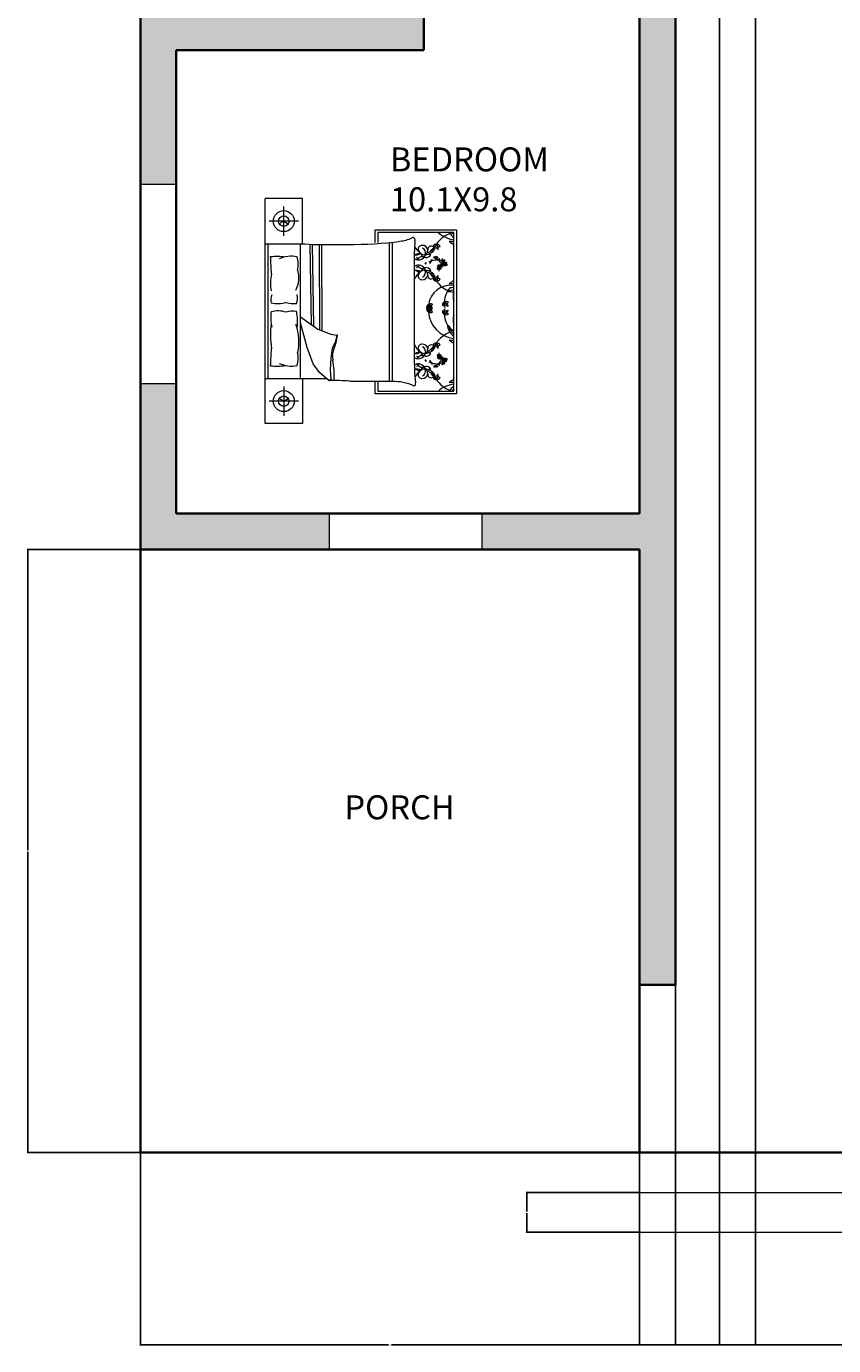
# Model space of a CAD drawing. Units: inches. Extents: x 8 to 486, y -516 to 97.
# Tile 1 of 5: x 9 to 211, y -516 to -185. Entities that reach past the tile are written whole.
import ezdxf

# ---------------------------------------------------------------- set-up
doc = ezdxf.new("R2010")
doc.units = ezdxf.units.IN
doc.header["$MEASUREMENT"] = 0
for name, color, linetype, lineweight in [('A-ANNO-DIMS', 2, 'Continuous', 18), ('A-AREA-IDEN', 7, 'Continuous', 18), ('A-FLOR-STRS', 7, 'Continuous', 18), ('A-FURN', 8, 'Continuous', 18), ('A-GLAZ', 4, 'Continuous', 18), ('A-WALL', 7, 'Continuous', 35), ('A-WALL-PATT', 150, 'Continuous', 13)]:
    doc.layers.add(name, color=color, linetype=linetype, lineweight=lineweight)
doc.styles.get("Standard").update_dxf_attribs({"font": 'arial.ttf'})
doc.dimstyles.get("Standard").update_dxf_attribs({"dimtxt": 0.18, "dimasz": 0.18, "dimexe": 0.18, "dimexo": 0.0625, "dimgap": 0.09, "dimtad": 0, "dimtih": 1, "dimtoh": 1, "dimdec": 0, "dimzin": 0, "dimdsep": 46, "dimlunit": 3, "dimtxsty": 'Standard', "dimcen": 0.09, "dimadec": 0, "dimazin": 0, "dimtfac": 1, "dimtdec": 0, "dimtofl": 0, "dimtmove": 0, "dimatfit": 3, "dimfxl": 1, "dimtolj": 1, "dimtzin": 0, "dimarcsym": 0})

# ---------------------------------------------------------------- blocks, each defined once
blk = doc.blocks.new('BED-DOUBLE')
for p, q in [((0, 0), (0, 56.34)), ((4.7, 47.03), (4.7, 54.39)), ((8.38, 50.71), (1.01, 50.71)), ((27.62, 45.39), (27.62, 48.51)), ((27.62, 48.51), (47.92, 48.51)), ((28.27, 47.86), (28.27, 45.37)), ((47.26, 47.86), (28.27, 47.86)), ((47.26, 8.09), (47.26, 47.86)), ((47.92, 48.51), (47.92, 7.44)), ((0.72, 45.07), (0.72, 11.27)), ((8.9, 11.27), (8.9, 45.07)), ((11.24, 44.92), (11.53, 24.86)), ((11.82, 44.9), (12.11, 24.44)), ((13.6, 44.87), (13.68, 23.48)), ((14.18, 44.87), (14.26, 23.26)), ((31.13, 45.33), (31.13, 10.62)), ((31.84, 45.38), (31.84, 10.62)), ((41.55, 42.31), (40.91, 42.43)), ((37.37, 39.61), (37.37, 16.73)), ((41.55, 38.37), (40.91, 38.24)), ((8.9, 26.75), (13.2, 23.66)), ((10.58, 19.09), (8.9, 25.24)), ((13.2, 23.66), (16.51, 22.4)), ((16.51, 22.4), (17.99, 22.17)), ((17.54, 20.35), (16.85, 18.87)), ((17.99, 22.17), (17.54, 20.35)), ((12.06, 14.99), (10.58, 19.09)), ((16.85, 18.87), (16.51, 16.36)), ((41.55, 17.58), (40.91, 17.7)), ((13.66, 12.82), (12.06, 14.99)), ((16.51, 16.36), (16.28, 13.5)), ((16.28, 13.5), (16.51, 11.22)), ((41.55, 13.64), (40.91, 13.52)), ((0, 11.27), (15.46, 11.27)), ((16.05, 10.76), (13.66, 12.82)), ((16.51, 11.22), (16.05, 10.76)), ((27.62, 7.44), (27.62, 10.62)), ((28.27, 10.62), (28.27, 8.09)), ((4.7, 9.31), (4.7, 1.95)), ((47.92, 7.44), (27.62, 7.44)), ((28.27, 8.09), (47.26, 8.09)), ((8.38, 5.63), (1.01, 5.63))]:
    blk.add_line(p, q)
for points in [[(0, 45.07), (9.39, 45.07), (9.39, 56.34), (0, 56.34)], [(4.7, 50.71), (3.56, 50.05)], [(4.7, 50.71), (5.83, 50.05)], [(9.39, 11.27), (9.39, 0), (0, 0)], [(4.7, 5.63), (3.56, 6.29)], [(4.7, 5.63), (5.83, 6.29)]]:
    blk.add_lwpolyline(points)
for points in [[(30.69, 45.31, 0.056112), (33.79, 45.72, 0.095341), (36.78, 46.51)], [(1.4, 41.84, -0.074897), (5.08, 41.77, 0.472817)], [(5.29, 30.31, -0.14099), (1.54, 30.2, -0.235245)], [(5.29, 27.91, 0.14099), (1.54, 28.02, 0.235245)], [(1.4, 14.5, 0.074897), (5.08, 14.57, -0.472817)], [(21.21, 10.65, 0.001242), (31.9, 10.62, -0.127202), (37.23, 9.49)]]:
    blk.add_lwpolyline(points, format="xyb")
for centre, radius in [((4.7, 50.71), 2.63), ((4.7, 50.71), 1.31), ((45.1, 39.99), 0.143), ((43.59, 39.05), 0.143), ((43.59, 16.9), 0.143), ((45.1, 15.96), 0.143), ((4.7, 5.63), 2.63), ((4.7, 5.63), 1.31)]:
    blk.add_circle(centre, radius)
for centre, radius, start, end in [((37.06, 46.09), 0.514, 336.5219, 123.8264), ((48.98, 40.75), 7.36, 111.4092, 145.6135), ((48.25, 53.34), 7.36, 228.1144, 262.255), ((49.24, 49.64), 3.59, 209.8884, 236.5383), ((49.91, 50.93), 4.47, 223.5186, 233.6964), ((15.79, 146.07), 101.24, 266.1, 270.9282), ((19.47, 176.89), 132.06, 269.1145, 274.8735), ((92.17, 41.33), 54.82, 175.2402, 181.8035), ((41.34, 46.16), 4.26, 203.6453, 236.3329), ((39.29, 43.68), 0.951, 88.9462, 185.5144), ((39.99, 43.97), 1.69, 193.079, 274.7067), ((39.43, 43.29), 1.35, 7.1143, 95.0551), ((38.92, 42.76), 1.31, 338.5779, 68.4181), ((39.13, 43.52), 1.64, 305.9599, 357.6409), ((39.73, 45.27), 2.66, 288.2955, 328.7386), ((41.6, 43.6), 0.846, 19.1312, 189.736), ((41.34, 43.8), 1.06, 285.6955, 4.031), ((42.75, 42.66), 1.12, 128.4175, 173.8338), ((42.51, 43.77), 0.518, 126.7319, 206.0245), ((42.76, 44.31), 0.61, 76.272, 177.0484), ((41.84, 45.56), 1.26, 284.7031, 328.6173), ((43.59, 43.96), 1.16, 125.7657, 194.5347), ((37.88, 46.02), 5.15, 332.8176, 347.4827), ((43.08, 44.11), 0.816, 20.9613, 102.2885), ((43.52, 44.92), 0.614, 181.7131, 301.5367), ((41.51, 43.68), 1.86, 2.0648, 41.1598), ((42.63, 44.37), 0.602, 316.2238, 62.3173), ((42.98, 44.02), 0.048, 20.2667, 316.2271), ((43.23, 43.75), 0.0444, 52.0591, 168.5166), ((43.28, 43.74), 0.0914, 168.5166, 2.0648), ((48.41, 47.64), 2.99, 221.0454, 247.4453), ((46.8, 55.83), 10.18, 266.3481, 272.5919), ((-534.78, 10.78), 537.08, 2.8502, 3.3148), ((6.56, 34.66), 7.26, 78.2417, 114.8684), ((0.75, 39.83), 7.55, 348.9631, 14.8961), ((37.99, 41.7), 0.679, 196.6343, 225.5483), ((37.79, 44.6), 2.33, 259.249, 301.1782), ((37.99, 41.7), 0.679, 127.675, 162.5814), ((38.39, 42.79), 1.8, 240.8249, 340.7178), ((37.86, 41.99), 0.843, 246.1646, 318.4347), ((38.39, 37.89), 1.8, 19.2822, 119.1751), ((38.8, 40.44), 2.17, 85.2696, 124.215), ((38.72, 43.06), 1.62, 240.0851, 262.564), ((39.35, 40.67), 1.16, 74.8529, 138.4347), ((40.34, 43), 1.4, 196.8663, 330.0915), ((39.75, 42.12), 0.35, 254.8529, 12.6959), ((38.8, 40.44), 2.17, 53.6555, 57.2989), ((40.21, 40.19), 0.177, 169.5864, 349.5616), ((39.95, 45.3), 3.02, 273.4924, 303.7117), ((40.28, 40.18), 0.109, 349.5616, 167.2949), ((43.11, 36.27), 4.67, 110.1059, 116.9968), ((41.55, 40.12), 0.296, 129.5056, 182.6421), ((40.7, 40.8), 0.89, 308.4388, 328.836), ((40.54, 41.53), 1.59, 296.5064, 305.3102), ((40.53, 40.71), 0.905, 336.3901, 344.4871), ((41.52, 40.48), 0.115, 83.9457, 185.6216), ((41.06, 40.58), 0.472, 328.836, 0.8141), ((41.3, 40.45), 0.27, 306.5232, 32.4668), ((41.62, 40.66), 0.115, 112.5583, 214.2343), ((41.55, 40.86), 0.27, 265.7131, 351.6568), ((41.31, 41.01), 0.472, 297.3659, 329.344), ((40.95, 41.42), 0.905, 313.6929, 321.7899), ((41.96, 40.8), 0.296, 115.5379, 168.6744), ((40.95, 41.22), 0.89, 329.344, 349.7412), ((43.11, 36.27), 4.67, 86.1723, 106.4158), ((40.24, 41.02), 1.59, 352.8698, 1.6736), ((42.35, 41.59), 0.111, 125.0752, 284.7644), ((42.52, 41.63), 0.239, 127.3642, 168.4363), ((42.33, 41.83), 0.345, 277.4968, 341.2737), ((42.6, 41.67), 0.137, 88.1325, 178.8919), ((42.88, 41.52), 0.297, 136.3462, 189.6513), ((42.71, 41.49), 0.124, 189.6513, 312.3208), ((42.74, 41.83), 0.143, 183.2768, 356.7232), ((43.19, 41.58), 0.47, 164.2829, 186.9148), ((42.63, 41.57), 0.235, 312.3208, 40.2111), ((43.13, 41.84), 0.333, 201.6382, 274.947), ((42.69, 41.38), 0.436, 42.3896, 66.5724), ((47.08, 44.83), 5.35, 217.9541, 226.8459), ((43, 41.64), 0.237, 10.9597, 52.2379), ((43.15, 41.62), 0.11, 274.947, 37.5263), ((43.38, 40.15), 0.654, 253.6301, 325.4631), ((43.56, 39.24), 0.463, 82.0748, 142.6895), ((43.52, 40.99), 0.115, 112.5583, 214.2343), ((43.45, 41.2), 0.27, 265.7131, 351.6568), ((43.21, 41.35), 0.472, 297.3659, 329.344), ((43.23, 38.6), 2.34, 60.7959, 85.244), ((38.25, 35.23), 7.7, 37.8256, 47.7588), ((42.85, 41.75), 0.905, 313.6929, 321.7899), ((43.52, 39.8), 0.398, 273.8774, 357.1501), ((43.85, 41.13), 0.296, 115.5379, 168.6744), ((42.85, 41.56), 0.89, 329.344, 349.7412), ((43.68, 40.08), 0.385, 262.0748, 308.2393), ((42.14, 41.35), 1.59, 352.8698, 1.6736), ((44.3, 39.69), 0.398, 181.4625, 249.4747), ((46.34, 38.35), 2.81, 130.182, 149.456), ((44.23, 40), 0.385, 215.1128, 261.2773), ((44.54, 39.98), 0.654, 197.889, 269.722), ((44.37, 41.03), 0.16, 33.0979, 123.1364), ((40.84, 38.77), 4.19, 31.1156, 34.8118), ((44.14, 40.76), 0.434, 2.3172, 70.5201), ((44.79, 39.95), 0.463, 139.3812, 199.9959), ((43.93, 40.29), 0.654, 310.9365, 22.7695), ((44.23, 40.25), 0.475, 285.6484, 332.2957), ((44.5, 40.65), 0.125, 135.7354, 318.1297), ((44.29, 40.86), 0.166, 315.7354, 31.1156), ((44.15, 40.5), 0.385, 319.3812, 5.5456), ((44.59, 40.65), 0.125, 68.2452, 250.6395), ((44.3, 40.81), 0.374, 352.6008, 57.1845), ((45.64, 38.3), 2.5, 111.7087, 116.2181), ((43.23, 38.6), 2.34, 47.5083, 55.9967), ((44.66, 40.89), 0.374, 252.8042, 349.6943), ((44.3, 40.22), 0.398, 331.1838, 51.6792), ((44.71, 39.75), 0.111, 125.0752, 284.7644), ((44.7, 40.92), 0.166, 248.2452, 323.6254), ((44.88, 39.79), 0.239, 93.635, 168.4363), ((44.55, 41.02), 0.434, 291.7087, 3.0299), ((44.85, 40.17), 0.141, 138.2946, 276.2474), ((44.69, 39.98), 0.345, 277.4968, 341.2737), ((44.9, 40.15), 0.196, 358.5719, 143.8954), ((41.46, 43.31), 4.19, 323.6254, 327.3216), ((44.97, 39.82), 0.137, 88.1325, 178.8919), ((45.02, 40.3), 0.197, 208.8493, 269.9355), ((44.85, 40.26), 0.226, 274.2123, 318.1587), ((45.24, 39.68), 0.297, 136.3462, 189.6513), ((44.89, 40.92), 0.16, 325.6077, 55.6462), ((45.55, 39.73), 0.47, 164.2829, 186.9148), ((45.54, 40.03), 0.452, 121.9501, 165.2442), ((45, 39.73), 0.235, 312.3208, 40.2111), ((45.5, 39.99), 0.333, 201.6382, 274.947), ((45.23, 40.2), 0.095, 262.868, 7.094), ((45.05, 39.54), 0.436, 42.3896, 66.5724), ((45.21, 40.28), 0.283, 278.5614, 22.5914), ((45.37, 39.79), 0.237, 10.9597, 118.7804), ((45.37, 40.29), 0.142, 44.3732, 121.9501), ((45.52, 39.77), 0.11, 274.947, 37.5263), ((11.26, 35.15), 9.9, 166.3427, 191.1841), ((1.3, 36.57), 7.17, 333.8761, 16.1746), ((37.99, 38.97), 0.679, 134.4517, 156.7144), ((37.99, 38.97), 0.679, 203.2856, 232.325), ((37.79, 36.08), 2.33, 58.8218, 100.2867), ((41.34, 34.52), 4.26, 123.6671, 158.5059), ((37.86, 38.68), 0.843, 41.5653, 113.8354), ((38.8, 40.23), 2.17, 235.785, 274.7304), ((38.72, 37.62), 1.62, 97.436, 119.9149), ((39.99, 36.71), 1.69, 85.2933, 166.921), ((39.29, 37), 0.951, 174.4856, 271.0538), ((39.35, 40.01), 1.16, 221.5653, 285.1471), ((40.34, 37.67), 1.4, 29.9085, 163.1337), ((39.43, 37.39), 1.35, 264.9449, 352.8857), ((38.92, 37.92), 1.31, 291.5819, 21.4221), ((39.75, 38.56), 0.35, 347.3041, 105.1471), ((38.8, 40.23), 2.17, 302.7011, 306.3445), ((39.13, 37.16), 1.64, 2.3591, 54.0401), ((39.95, 35.38), 3.02, 56.2883, 86.5076), ((39.73, 35.4), 2.66, 31.2614, 71.7045), ((41.6, 37.08), 0.846, 170.264, 340.8688), ((42.75, 38.01), 1.12, 186.1662, 231.5825), ((41.34, 36.88), 1.06, 355.969, 74.3045), ((42.51, 36.91), 0.518, 153.9755, 233.2681), ((43.59, 36.72), 1.16, 165.4653, 234.2343), ((37.88, 34.66), 5.15, 12.5173, 27.1824), ((41.51, 37), 1.86, 318.8402, 357.9352), ((42.63, 36.3), 0.602, 297.6827, 43.7762), ((43.52, 35.75), 0.614, 58.4633, 178.2869), ((43.01, 36.67), 0.0796, 43.7762, 339.7183), ((43.2, 38.81), 0.111, 125.0752, 284.7644), ((43.37, 38.85), 0.239, 93.635, 168.4363), ((43.51, 39.88), 0.475, 228.342, 274.9894), ((43.28, 36.93), 0.0914, 357.9352, 191.4834), ((43.23, 36.92), 0.0444, 191.4834, 307.9409), ((43.34, 39.23), 0.141, 138.2946, 276.2474), ((43.39, 39.21), 0.196, 358.5719, 143.8954), ((43.18, 39.05), 0.345, 277.4968, 341.2737), ((43.46, 38.88), 0.137, 88.1325, 178.8919), ((43.51, 39.36), 0.197, 208.8493, 269.9355), ((43.34, 39.32), 0.226, 274.2123, 318.1587), ((43.73, 38.74), 0.297, 136.3462, 189.6513), ((43.56, 38.71), 0.124, 189.6513, 312.3208), ((46.34, 38.35), 2.81, 175.2415, 182.8929), ((44.04, 38.79), 0.47, 164.2829, 186.9148), ((44.03, 39.09), 0.452, 121.9501, 165.2442), ((43.49, 38.79), 0.235, 312.3208, 40.2111), ((43.98, 39.06), 0.333, 201.6382, 274.947), ((43.71, 39.26), 0.095, 262.868, 7.094), ((43.54, 38.6), 0.436, 42.3896, 66.5724), ((43.7, 39.34), 0.283, 278.5614, 22.5914), ((43.86, 38.86), 0.237, 10.9597, 118.7804), ((46.34, 38.35), 2.81, 156.1523, 156.9499), ((43.86, 39.35), 0.142, 44.3732, 121.9501), ((44, 38.83), 0.11, 274.947, 37.5263), ((44.34, 39.76), 0.475, 248.3627, 295.0101), ((44.1, 39.16), 0.463, 20.6625, 81.2773), ((45.07, 39.65), 0.124, 189.6513, 312.3208), ((46.55, 28.98), 5.69, 82.8636, 171.8197), ((42.76, 36.36), 0.61, 182.9516, 283.728), ((41.84, 35.12), 1.26, 31.3827, 75.2969), ((43.08, 36.57), 0.816, 257.7115, 339.0387), ((48.98, 39.93), 7.36, 214.3865, 248.5908), ((52.19, 29.78), 7.36, 152.5854, 175.5377), ((46.95, 32.74), 1.32, 76.3898, 169.0739), ((46.77, 31.74), 1.67, 72.8609, 131.9049), ((48.41, 33.04), 2.99, 112.5547, 138.9546), ((46.8, 24.84), 10.18, 87.4081, 93.6519), ((4.21, 30.97), 2.79, 153.3437, 196.1026), ((7.17, 36.95), 6.9, 254.1707, 275.9871), ((5.19, 31.35), 2.99, 335.0183, 18.5407), ((41.09, 29.2), 0.61, 106.1963, 206.9726), ((39.66, 29.82), 1.26, 314.6273, 358.5415), ((41.98, 29.31), 1.16, 155.6899, 224.4589), ((41.47, 29.19), 0.816, 50.8855, 132.2127), ((41.44, 30.11), 0.614, 211.6373, 331.4609), ((40.94, 29.19), 0.602, 346.148, 92.2415), ((40.32, 28.03), 1.86, 31.989, 71.0841), ((36.01, 28.25), 5.15, 2.7418, 17.407), ((45.03, 29.77), 0.61, 106.1963, 206.9726), ((43.6, 30.38), 1.26, 314.6273, 358.5415), ((45.92, 29.87), 1.16, 155.6899, 224.4589), ((45.41, 29.75), 0.816, 50.8855, 132.2127), ((45.38, 30.68), 0.614, 211.6373, 331.4609), ((44.26, 28.59), 1.86, 31.989, 71.0841), ((39.95, 28.81), 5.15, 2.7418, 17.407), ((44.88, 29.75), 0.602, 346.148, 92.2415), ((46.03, 29.72), 3.29, 68.117, 96.6195), ((51.13, 31.84), 4.05, 162.9798, 196.4569), ((53.22, 30.24), 5.98, 174.3643, 175.6213), ((57.31, 27.08), 10.69, 160.0972, 160.2783), ((11.47, 26.54), 10.04, 171.5249, 193.96), ((7.17, 21.26), 6.9, 84.0129, 105.8293), ((-1.76, 25.79), 9.94, 349.8617, 13.6238), ((41.09, 28.62), 0.61, 153.0274, 253.8037), ((39.66, 28), 1.26, 1.4585, 45.3727), ((41.98, 28.51), 1.16, 135.5411, 204.3101), ((36.01, 29.58), 5.15, 342.593, 357.2582), ((40.32, 29.8), 1.86, 288.9159, 328.011), ((40.94, 28.64), 0.602, 267.7585, 13.852), ((41.44, 27.71), 0.614, 28.5391, 148.3627), ((41.47, 28.64), 0.816, 227.7873, 309.1145), ((48.25, 28.61), 7.36, 184.4623, 262.255), ((41.42, 29.06), 0.048, 50.1909, 346.0209), ((41.45, 28.76), 0.0796, 13.852, 309.9245), ((41.82, 28.97), 0.0914, 198.4408, 31.989), ((41.77, 28.95), 0.0444, 81.9833, 198.4408), ((41.82, 28.86), 0.0914, 328.011, 161.5592), ((41.77, 28.87), 0.0444, 161.5592, 278.0167), ((45.03, 28.06), 0.61, 153.0274, 253.8037), ((43.6, 27.44), 1.26, 1.4585, 45.3727), ((45.92, 27.95), 1.16, 135.5411, 204.3101), ((39.95, 29.01), 5.15, 342.593, 357.2582), ((44.26, 29.23), 1.86, 288.9159, 328.011), ((44.88, 28.07), 0.602, 267.7585, 13.852), ((45.38, 27.15), 0.614, 28.5391, 148.3627), ((45.41, 28.08), 0.816, 227.7873, 309.1145), ((52.19, 28.04), 7.36, 184.4623, 207.4146), ((45.36, 29.62), 0.048, 50.1909, 346.0209), ((45.39, 28.2), 0.0796, 13.852, 309.9245), ((45.76, 29.53), 0.0914, 198.4408, 31.989), ((45.71, 29.52), 0.0444, 81.9833, 198.4408), ((45.76, 28.3), 0.0914, 328.011, 161.5592), ((45.71, 28.31), 0.0444, 161.5592, 278.0167), ((51.13, 25.99), 4.05, 163.5431, 197.0202), ((53.22, 27.59), 5.98, 184.3787, 185.6357), ((57.31, 30.74), 10.69, 199.7217, 199.9028), ((21.79, 22.22), 20.43, 172.2196, 189.497), ((-4.62, 20.49), 13.1, 348.0397, 19.2615), ((49.24, 24.92), 3.59, 181.272, 236.5383), ((51.16, 28.56), 6.65, 214.0123, 234.053), ((49.91, 26.21), 4.47, 197.8504, 233.6964), ((-3.3, 26.09), 21.85, 340.1194, 349.3383), ((18.04, 22.05), 0.136, 358.8623, 109.7536), ((41.34, 21.43), 4.26, 201.4941, 236.3329), ((39.29, 18.95), 0.951, 88.9462, 185.5144), ((39.43, 18.56), 1.35, 7.1143, 95.0551), ((42.76, 19.58), 0.61, 76.272, 177.0484), ((41.84, 20.83), 1.26, 284.7031, 328.6173), ((43.59, 19.23), 1.16, 125.7657, 194.5347), ((37.88, 21.29), 5.15, 332.8176, 347.4827), ((48.98, 16.02), 7.36, 111.4092, 145.6135), ((43.08, 19.38), 0.816, 20.9613, 102.2885), ((42.63, 19.64), 0.602, 316.2238, 62.3173), ((41.51, 18.95), 1.86, 2.0648, 41.1598), ((43.52, 20.19), 0.614, 181.7131, 301.5367), ((46.8, 31.1), 10.18, 266.3481, 272.5919), ((48.41, 22.91), 2.99, 221.0454, 247.4453), ((-534.78, 45.56), 537.08, 356.6852, 357.1498), ((0.75, 16.51), 7.55, 345.1039, 11.0369), ((21.45, 16.81), 4.59, 156.2616, 191.3392), ((37.79, 19.87), 2.33, 259.7133, 301.1782), ((37.99, 16.98), 0.679, 127.675, 156.7144), ((96.02, 16.06), 58.65, 179.3433, 185.6887), ((37.99, 16.98), 0.679, 203.229, 225.5483), ((38.39, 18.06), 1.8, 240.8249, 340.7178), ((37.86, 17.26), 0.843, 246.1646, 318.4347), ((38.8, 15.72), 2.17, 85.2696, 124.215), ((38.72, 18.33), 1.62, 240.0851, 262.564), ((39.99, 19.24), 1.69, 193.079, 274.7067), ((39.35, 15.94), 1.16, 74.8529, 138.4347), ((40.34, 18.28), 1.4, 196.8663, 330.0915), ((38.92, 18.03), 1.31, 338.5779, 68.4181), ((39.75, 17.39), 0.35, 254.8529, 12.6959), ((38.8, 15.72), 2.17, 53.6555, 57.2989), ((39.13, 18.79), 1.64, 305.9599, 357.6409), ((39.95, 20.57), 3.02, 273.4924, 303.7117), ((39.73, 20.54), 2.66, 288.2955, 328.7386), ((41.6, 18.87), 0.846, 19.1312, 189.736), ((41.34, 19.07), 1.06, 285.6955, 4.031), ((42.75, 17.93), 1.12, 128.4175, 173.8338), ((42.51, 19.04), 0.518, 126.7319, 206.0245), ((42.98, 19.29), 0.048, 20.2667, 316.2271), ((43.2, 17.14), 0.111, 75.2356, 234.9248), ((43.37, 17.09), 0.239, 191.5637, 266.365), ((43.23, 19.02), 0.0444, 52.0591, 168.5166), ((43.28, 19.02), 0.0914, 168.5166, 2.0648), ((43.51, 16.07), 0.475, 85.0106, 131.658), ((43.34, 16.72), 0.141, 83.7526, 221.7054), ((43.18, 16.9), 0.345, 18.7263, 82.5032), ((43.39, 16.74), 0.196, 216.1046, 1.4281), ((43.46, 17.06), 0.137, 181.1081, 271.8675), ((43.51, 16.58), 0.197, 90.0645, 151.1507), ((43.34, 16.63), 0.226, 41.8413, 85.7877), ((43.73, 17.21), 0.297, 170.3487, 223.6538), ((43.56, 17.24), 0.124, 47.6792, 170.3487), ((46.34, 17.59), 2.81, 177.1071, 184.7585), ((43.52, 16.15), 0.398, 2.8499, 86.1226), ((44.04, 17.15), 0.47, 173.0852, 195.7171), ((44.03, 16.86), 0.452, 194.7558, 238.0499), ((43.49, 17.16), 0.235, 319.7889, 47.6792), ((43.98, 16.89), 0.333, 85.053, 158.3618), ((43.71, 16.68), 0.095, 352.906, 97.132), ((43.54, 17.35), 0.436, 293.4276, 317.6104), ((43.86, 17.09), 0.237, 241.2196, 349.0403), ((43.7, 16.6), 0.283, 337.4086, 81.4386), ((44.3, 16.26), 0.398, 110.5253, 178.5375), ((44.54, 15.97), 0.654, 90.278, 162.111), ((44, 17.11), 0.11, 322.4737, 85.053), ((44.34, 16.19), 0.475, 64.9899, 111.6373), ((44.1, 16.78), 0.463, 278.7227, 339.3375), ((6.56, 21.68), 7.26, 245.1316, 281.7583), ((-3.9, 11.73), 21.26, 357.4519, 11.3392), ((37.99, 14.24), 0.679, 134.4517, 153.558), ((37.99, 14.24), 0.679, 210.0293, 232.325), ((37.79, 11.35), 2.33, 58.8218, 99.1554), ((38.39, 13.16), 1.8, 19.2822, 119.1751), ((37.86, 13.96), 0.843, 41.5653, 113.8354), ((41.34, 9.79), 4.26, 123.6671, 153.2997), ((38.8, 15.5), 2.17, 235.785, 274.7304), ((38.72, 12.89), 1.62, 97.436, 119.9149), ((39.99, 11.98), 1.69, 85.2933, 166.921), ((39.35, 15.28), 1.16, 221.5653, 285.1471), ((40.34, 12.94), 1.4, 29.9085, 163.1337), ((38.92, 13.19), 1.31, 291.5819, 21.4221), ((39.75, 13.83), 0.35, 347.3041, 105.1471), ((38.8, 15.5), 2.17, 302.7011, 306.3445), ((40.21, 15.76), 0.177, 10.4384, 190.4136), ((39.13, 12.43), 1.64, 2.3591, 54.0401), ((39.95, 10.65), 3.02, 56.2883, 86.5076), ((40.28, 15.77), 0.109, 192.7051, 10.4384), ((43.11, 19.68), 4.67, 243.0032, 249.8941), ((40.7, 15.15), 0.89, 31.164, 51.5612), ((41.55, 15.83), 0.296, 177.3579, 230.4944), ((40.54, 14.42), 1.59, 54.6898, 63.4936), ((40.53, 15.24), 0.905, 15.5129, 23.6099), ((41.52, 15.47), 0.115, 174.3784, 276.0543), ((41.3, 15.5), 0.27, 327.5332, 53.4768), ((41.06, 15.36), 0.472, 359.1859, 31.164), ((41.62, 15.29), 0.115, 145.7657, 247.4417), ((41.55, 15.09), 0.27, 8.3432, 94.2869), ((41.31, 14.94), 0.472, 30.656, 62.6341), ((40.95, 14.53), 0.905, 38.2101, 46.3071), ((41.96, 15.15), 0.296, 191.3256, 244.4621), ((40.95, 14.72), 0.89, 10.2588, 30.656), ((43.11, 19.68), 4.67, 253.5842, 273.8277), ((40.24, 14.93), 1.59, 358.3264, 7.1302), ((42.35, 14.36), 0.111, 75.2356, 234.9248), ((42.52, 14.31), 0.239, 191.5637, 232.6358), ((42.33, 14.12), 0.345, 18.7263, 82.5032), ((42.6, 14.28), 0.137, 181.1081, 271.8675), ((42.88, 14.43), 0.297, 170.3487, 223.6538), ((42.71, 14.46), 0.124, 47.6792, 170.3487), ((42.74, 14.11), 0.143, 3.2768, 176.7232), ((43.19, 14.37), 0.47, 173.0852, 195.7171), ((42.63, 14.37), 0.235, 319.7889, 47.6792), ((43.13, 14.11), 0.333, 85.053, 158.3618), ((42.69, 14.57), 0.436, 293.4276, 317.6104), ((47.08, 11.12), 5.35, 133.1541, 142.0459), ((43, 14.31), 0.237, 307.7621, 349.0403), ((43.15, 14.33), 0.11, 322.4737, 85.053), ((43.38, 15.8), 0.654, 34.5369, 106.3699), ((43.56, 16.71), 0.463, 217.3105, 277.9252), ((43.52, 14.96), 0.115, 145.7657, 247.4417), ((38.25, 20.72), 7.7, 312.2412, 322.1744), ((43.23, 17.35), 2.34, 274.756, 299.2041), ((43.45, 14.75), 0.27, 8.3432, 94.2869), ((43.21, 14.6), 0.472, 30.656, 62.6341), ((42.85, 14.2), 0.905, 38.2101, 46.3071), ((43.85, 14.81), 0.296, 191.3256, 244.4621), ((42.85, 14.39), 0.89, 10.2588, 30.656), ((43.68, 15.87), 0.385, 51.7607, 97.9252), ((42.14, 14.59), 1.59, 358.3264, 7.1302), ((46.34, 17.59), 2.81, 203.0501, 203.8477), ((43.86, 16.59), 0.142, 238.0499, 315.6268), ((44.23, 15.95), 0.385, 98.7227, 144.8872), ((46.34, 17.59), 2.81, 210.544, 229.818), ((44.14, 15.19), 0.434, 289.4799, 357.6828), ((40.84, 17.17), 4.19, 325.1882, 328.8844), ((44.37, 14.91), 0.16, 236.8636, 326.9021), ((44.79, 15.99), 0.463, 160.0041, 220.6188), ((43.93, 15.66), 0.654, 337.2305, 49.0635), ((44.23, 15.7), 0.475, 27.7043, 74.3516), ((44.5, 15.3), 0.125, 41.8703, 224.2646), ((44.29, 15.09), 0.166, 328.8844, 44.2646), ((44.15, 15.44), 0.385, 354.4544, 40.6188), ((44.59, 15.29), 0.125, 109.3605, 291.7548), ((44.3, 15.14), 0.374, 302.8155, 7.3992), ((45.64, 17.65), 2.5, 243.7819, 248.2913), ((43.23, 17.35), 2.34, 304.0033, 312.4917), ((44.3, 15.72), 0.398, 308.3208, 28.8162), ((44.66, 15.06), 0.374, 10.3057, 107.1958), ((44.71, 16.2), 0.111, 75.2356, 234.9248), ((44.7, 15.02), 0.166, 36.3746, 111.7548), ((44.88, 16.16), 0.239, 191.5637, 266.365), ((44.85, 15.78), 0.141, 83.7526, 221.7054), ((44.55, 14.92), 0.434, 356.9701, 68.2913), ((44.69, 15.96), 0.345, 18.7263, 82.5032), ((44.9, 15.8), 0.196, 216.1046, 1.4281), ((44.97, 16.12), 0.137, 181.1081, 271.8675), ((41.46, 12.64), 4.19, 32.6784, 36.3746), ((45.02, 15.65), 0.197, 90.0645, 151.1507), ((44.85, 15.69), 0.226, 41.8413, 85.7877), ((45.07, 16.3), 0.124, 47.6792, 170.3487), ((45.24, 16.27), 0.297, 170.3487, 223.6538), ((44.89, 15.03), 0.16, 304.3538, 34.3923), ((45.55, 16.21), 0.47, 173.0852, 195.7171), ((45.54, 15.92), 0.452, 194.7558, 238.0499), ((45, 16.22), 0.235, 319.7889, 47.6792), ((45.5, 15.95), 0.333, 85.053, 158.3618), ((45.23, 15.75), 0.095, 352.906, 97.132), ((45.05, 16.41), 0.436, 293.4276, 317.6104), ((45.37, 16.15), 0.237, 241.2196, 349.0403), ((45.21, 15.67), 0.283, 337.4086, 81.4386), ((45.37, 15.66), 0.142, 238.0499, 315.6268), ((45.52, 16.18), 0.11, 322.4737, 85.053), ((17.45, -40.9), 51.68, 85.8294, 91.553), ((37.19, 10.01), 0.52, 273.98, 27.3412), ((39.29, 12.27), 0.951, 174.4856, 271.0538), ((39.43, 12.66), 1.35, 264.9449, 352.8857), ((39.73, 10.68), 2.66, 31.2614, 71.7045), ((41.6, 12.35), 0.846, 170.264, 340.8688), ((41.34, 12.15), 1.06, 355.969, 74.3045), ((42.75, 13.29), 1.12, 186.1662, 231.5825), ((42.51, 12.18), 0.518, 153.9755, 233.2681), ((41.84, 10.39), 1.26, 31.3827, 75.2969), ((42.76, 11.64), 0.61, 182.9516, 283.728), ((43.59, 11.99), 1.16, 165.4653, 234.2343), ((37.88, 9.93), 5.15, 12.5173, 27.1824), ((41.51, 12.27), 1.86, 318.8402, 357.9352), ((42.63, 11.58), 0.602, 297.6827, 43.7762), ((43.52, 11.03), 0.614, 58.4633, 178.2869), ((43.08, 11.84), 0.816, 257.7115, 339.0387), ((48.98, 15.2), 7.36, 214.3865, 248.5908), ((43.01, 11.94), 0.0796, 43.7762, 339.7183), ((43.28, 12.2), 0.0914, 357.9352, 191.4834), ((43.23, 12.2), 0.0444, 191.4834, 307.9409), ((48.41, 8.31), 2.99, 112.5547, 138.9546), ((46.8, 0.12), 10.18, 87.4081, 93.6519), ((48.25, 2.61), 7.36, 97.745, 131.8856), ((49.24, 6.3), 3.59, 123.4617, 150.1116), ((49.91, 5.01), 4.47, 126.3036, 136.4814)]:
    blk.add_arc(centre, radius, start, end)
blk = doc.blocks.new('*D21')
at = {"layer": 'A-ANNO-DIMS', "color": 0, "lineweight": -2, "transparency": 16777216}
for p, q in [((37.13, -467.33), (37.13, -515.64)), ((162.13, -467.33), (162.13, -515.64)), ((37.31, -515.46), (99.24, -515.46)), ((161.95, -515.46), (100.02, -515.46))]:
    blk.add_line(p, q, dxfattribs=at)
at = {"layer": 'A-ANNO-DIMS', "color": 0, "transparency": 16777216}
for points in [[(37.31, -515.43), (37.31, -515.49), (37.13, -515.46)], [(161.95, -515.43), (161.95, -515.49), (162.13, -515.46)]]:
    blk.add_solid(points, dxfattribs=at)
at = {"layer": 'Defpoints', "color": 0, "transparency": 16777216}
for p in [(37.13, -467.26), (162.13, -467.26), (162.13, -515.46)]:
    blk.add_point(p, dxfattribs=at)
at = {"layer": 'A-ANNO-DIMS', "color": 0, "transparency": 16777216, "insert": (99.63, -515.46), "char_height": 0.18, "attachment_point": 5}
blk.add_mtext('\\A1;10\'-5"', dxfattribs=at)
blk = doc.blocks.new('*D22')
at = {"layer": 'A-ANNO-DIMS', "color": 0, "lineweight": -2, "transparency": 16777216}
for p, q in [((162.13, -487.33), (162.13, -515.64)), ((294.01, -487.33), (294.01, -515.64)), ((162.31, -515.46), (227.68, -515.46)), ((293.83, -515.46), (228.46, -515.46))]:
    blk.add_line(p, q, dxfattribs=at)
at = {"layer": 'A-ANNO-DIMS', "color": 0, "transparency": 16777216}
for points in [[(162.31, -515.43), (162.31, -515.49), (162.13, -515.46)], [(293.83, -515.43), (293.83, -515.49), (294.01, -515.46)]]:
    blk.add_solid(points, dxfattribs=at)
at = {"layer": 'Defpoints', "color": 0, "transparency": 16777216}
for p in [(162.13, -487.26), (294.01, -487.26), (294.01, -515.46)]:
    blk.add_point(p, dxfattribs=at)
at = {"layer": 'A-ANNO-DIMS', "color": 0, "transparency": 16777216, "insert": (228.07, -515.46), "char_height": 0.18, "attachment_point": 5}
blk.add_mtext('\\A1;11\'-0"', dxfattribs=at)
blk = doc.blocks.new('*D24')
at = {"layer": 'A-ANNO-DIMS', "color": 0, "lineweight": -2, "transparency": 16777216}
for p, q in [((37.06, -316.26), (8.75, -316.26)), ((8.93, -316.44), (8.93, -391.58)), ((8.93, -467.08), (8.93, -391.95)), ((37.06, -467.26), (8.75, -467.26))]:
    blk.add_line(p, q, dxfattribs=at)
at = {"layer": 'A-ANNO-DIMS', "color": 0, "transparency": 16777216}
for points in [[(8.9, -316.44), (8.96, -316.44), (8.93, -316.26)], [(8.9, -467.08), (8.96, -467.08), (8.93, -467.26)]]:
    blk.add_solid(points, dxfattribs=at)
at = {"layer": 'Defpoints', "color": 0, "transparency": 16777216}
for p in [(37.13, -316.26), (8.93, -467.26), (37.13, -467.26)]:
    blk.add_point(p, dxfattribs=at)
at = {"layer": 'A-ANNO-DIMS', "color": 0, "transparency": 16777216, "insert": (8.93, -391.76), "char_height": 0.18, "attachment_point": 5}
blk.add_mtext('\\A1;12\'-7"', dxfattribs=at)
blk = doc.blocks.new('*D26')
at = {"layer": 'A-ANNO-DIMS', "color": 0, "lineweight": -2, "transparency": 16777216}
for p, q in [((162.06, -477.26), (133.75, -477.26)), ((133.93, -477.44), (133.93, -482.08)), ((133.93, -487.08), (133.93, -482.45)), ((162.06, -487.26), (133.75, -487.26))]:
    blk.add_line(p, q, dxfattribs=at)
at = {"layer": 'A-ANNO-DIMS', "color": 0, "transparency": 16777216}
for points in [[(133.9, -477.44), (133.96, -477.44), (133.93, -477.26)], [(133.9, -487.08), (133.96, -487.08), (133.93, -487.26)]]:
    blk.add_solid(points, dxfattribs=at)
at = {"layer": 'Defpoints', "color": 0, "transparency": 16777216}
for p in [(133.93, -477.26), (162.13, -477.26), (162.13, -487.26)]:
    blk.add_point(p, dxfattribs=at)
at = {"layer": 'A-ANNO-DIMS', "color": 0, "transparency": 16777216, "insert": (133.93, -482.26), "char_height": 0.18, "attachment_point": 5}
blk.add_mtext('\\A1;0\'-10"', dxfattribs=at)
blk = doc.blocks.new('*D34')
at = {"layer": 'A-ANNO-DIMS', "color": 0, "lineweight": -2, "transparency": 16777216}
for p, q in [((171.13, -425.33), (171.13, -515.64)), ((233.38, -425.33), (233.38, -515.64)), ((171.31, -515.46), (201.92, -515.46)), ((233.2, -515.46), (202.58, -515.46))]:
    blk.add_line(p, q, dxfattribs=at)
at = {"layer": 'A-ANNO-DIMS', "color": 0, "transparency": 16777216}
for points in [[(171.31, -515.43), (171.31, -515.49), (171.13, -515.46)], [(233.2, -515.43), (233.2, -515.49), (233.38, -515.46)]]:
    blk.add_solid(points, dxfattribs=at)
at = {"layer": 'Defpoints', "color": 0, "transparency": 16777216}
for p in [(171.13, -425.26), (233.38, -425.26), (233.38, -515.46)]:
    blk.add_point(p, dxfattribs=at)
at = {"layer": 'A-ANNO-DIMS', "color": 0, "transparency": 16777216, "insert": (202.25, -515.46), "char_height": 0.18, "attachment_point": 5}
blk.add_mtext('\\A1;5\'-2"', dxfattribs=at)
blk = doc.blocks.new('*D35')
at = {"layer": 'A-ANNO-DIMS', "color": 0, "lineweight": -2, "transparency": 16777216}
for p, q in [((182.13, -73.93), (182.13, -515.64)), ((191.13, -73.93), (191.13, -515.64)), ((182.31, -515.46), (186.3, -515.46)), ((190.95, -515.46), (186.96, -515.46))]:
    blk.add_line(p, q, dxfattribs=at)
at = {"layer": 'A-ANNO-DIMS', "color": 0, "transparency": 16777216}
for points in [[(182.31, -515.43), (182.31, -515.49), (182.13, -515.46)], [(190.95, -515.43), (190.95, -515.49), (191.13, -515.46)]]:
    blk.add_solid(points, dxfattribs=at)
at = {"layer": 'Defpoints', "color": 0, "transparency": 16777216}
for p in [(182.13, -73.87), (191.13, -73.87), (191.13, -515.46)]:
    blk.add_point(p, dxfattribs=at)
at = {"layer": 'A-ANNO-DIMS', "color": 0, "transparency": 16777216, "insert": (186.63, -515.46), "char_height": 0.18, "attachment_point": 5}
blk.add_mtext('\\A1;0\'-9"', dxfattribs=at)

msp = doc.modelspace()

# ---------------------------------------------------------------- hatches: boundary and pattern name
at = {"layer": 'A-WALL-PATT'}
h = msp.add_hatch(color=256, dxfattribs=at)
h.dxf.hatch_style = 1
h.paths.add_polyline_path([(91.21, 12.74), (37.13, 12.74), (37.13, -29.65), (46.13, -29.65), (46.13, 3.74), (91.21, 3.74)])
h.paths.add_polyline_path([(211.13, 12.74), (137.85, 12.74), (137.85, 3.74), (182.13, 3.74), (182.13, -73.87), (191.13, -73.87), (191.13, 3.74), (211.13, 3.74)])
h.paths.add_polyline_path([(306.98, 12.74), (234.7, 12.74), (234.7, 3.74), (306.98, 3.74)])
h.paths.add_polyline_path([(267.13, 3.74), (258.13, 3.74), (258.13, -129.26), (267.13, -129.26)])
h.paths.add_polyline_path([(412.13, 12.74), (361.49, 12.74), (361.49, 3.74), (403.13, 3.74), (403.13, -35.28), (412.13, -35.28)])
h.paths.add_polyline_path([(379.01, -120.26), (297.29, -120.26), (297.29, -129.26), (325.13, -129.26), (325.13, -179.26), (218.14, -179.26), (218.14, -188.26), (325.13, -188.26), (325.13, -242.26), (297.29, -242.26), (297.29, -251.26), (379.01, -251.26), (379.01, -242.26), (334.13, -242.26), (334.13, -188.26), (403.13, -188.26), (403.13, -209.46), (412.13, -209.46), (412.13, -162.44), (403.13, -162.44), (403.13, -179.26), (334.13, -179.26), (334.13, -129.26), (379.01, -129.26)])
h.paths.add_polyline_path([(412.13, -70.38), (403.13, -70.38), (403.13, -142.55), (412.13, -142.55)])
h.paths.add_polyline_path([(412.13, -226.8), (403.13, -226.8), (403.13, -274.76), (412.13, -274.76)])
h.paths.add_polyline_path([(412.13, -317.95), (403.13, -317.95), (403.13, -361.26), (339.99, -361.26), (339.99, -370.26), (412.13, -370.26)])
h.paths.add_polyline_path([(412.13, -407.2), (403.13, -407.2), (403.13, -458.26), (373.42, -458.26), (373.42, -467.26), (412.13, -467.26)])
h.paths.add_polyline_path([(326.44, -458.26), (303.13, -458.26), (303.13, -283.74), (294.13, -283.74), (294.13, -416.26), (282.5, -416.26), (282.5, -425.26), (294.13, -425.26), (294.13, -467.26), (326.44, -467.26)])
h.paths.add_polyline_path([(246.84, -416.26), (233.38, -416.26), (233.38, -425.26), (246.84, -425.26)])
h.paths.add_polyline_path([(171.13, -307.26), (171.13, -191.26), (171.13, -182.26), (162.13, -182.26), (162.13, -191.26), (162.13, -307.26), (122.6, -307.26), (122.6, -316.26), (162.13, -316.26), (162.13, -425.26), (171.13, -425.26)])
h.paths.add_polyline_path([(84.39, -307.26), (46.13, -307.26), (46.13, -274.81), (37.13, -274.81), (37.13, -316.26), (84.39, -316.26)])
h.paths.add_polyline_path([(46.13, -191.26), (108.13, -191.26), (108.13, -182.26), (46.13, -182.26), (46.13, -172.25), (37.13, -172.25), (37.13, -224.84), (46.13, -224.84)])
h.paths.add_polyline_path([(191.13, -120.26), (46.13, -120.26), (46.13, -76.77), (37.13, -76.77), (37.13, -150.77), (46.13, -150.77), (46.13, -129.26), (99.13, -129.26), (99.13, -163.77), (108.13, -163.77), (108.13, -129.26), (191.13, -129.26)])

# ---------------------------------------------------------------- linework, layer by layer
at = {"layer": 'A-FLOR-STRS'}
for p, q in [((162.13, -467.26), (162.13, -477.26)), ((162.13, -477.26), (162.13, -487.26)), ((162.13, -477.26), (294.07, -477.26)), ((162.13, -487.26), (294.01, -487.26))]:
    msp.add_line(p, q, dxfattribs=at)
at = {"layer": 'A-GLAZ'}
for p, q in [((46.13, -224.84), (37.13, -224.84)), ((46.13, -274.81), (37.13, -274.81)), ((84.39, -307.26), (84.39, -316.26)), ((122.6, -307.26), (122.6, -316.26))]:
    msp.add_line(p, q, dxfattribs=at)
at = {"layer": 'A-WALL'}
for p, q in [((37.13, 12.74), (37.13, -467.26)), ((108.13, -182.26), (108.13, -191.26)), ((162.13, -191.26), (162.13, -182.26)), ((171.13, -191.26), (171.13, -182.26)), ((46.13, -191.26), (108.13, -191.26)), ((46.13, -191.26), (46.13, -307.26)), ((162.13, -191.26), (162.13, -307.26)), ((171.13, -191.26), (171.13, -425.26)), ((46.13, -307.26), (162.13, -307.26)), ((171.13, -307.26), (171.13, -425.26)), ((37.13, -316.26), (162.13, -316.26)), ((162.13, -316.26), (162.13, -467.26)), ((162.13, -425.26), (171.13, -425.26)), ((37.13, -467.26), (412.13, -467.26))]:
    msp.add_line(p, q, dxfattribs=at)

# ---------------------------------------------------------------- block references
at = {"layer": 'A-FURN'}
msp.add_blockref('BED-DOUBLE', (68.34, -284.75), dxfattribs=at)

# ---------------------------------------------------------------- texts
at = {"layer": 'A-AREA-IDEN', "insert": (99.61, -215.57), "char_height": 6, "attachment_point": 1}
msp.add_mtext('BEDROOM\\P10.1X9.8', dxfattribs=at)
at = {"layer": 'A-AREA-IDEN', "insert": (88.22, -377.83), "char_height": 6, "attachment_point": 1}
msp.add_mtext_dynamic_manual_height_columns('PORCH', width=0.3078, gutter_width=1, heights=[0], dxfattribs=at)

# ---------------------------------------------------------------- dimensions: what is measured, and where the dimension line sits
at = {"layer": 'A-ANNO-DIMS'}
for base, p1, p2, picture, middle in [((191.13, -515.46), (182.13, -73.87), (191.13, -73.87), '*D35', (186.63, -515.46)), ((233.3763, -515.4649), (171.1266, -425.2649), (233.3763, -425.2649), '*D34', (202.2515, -515.4649)), ((162.13, -515.46), (37.13, -467.26), (162.13, -467.26), '*D21', (99.63, -515.46)), ((294.01, -515.46), (162.13, -487.26), (294.01, -487.26), '*D22', (228.07, -515.46))]:
    dim = msp.add_linear_dim(base=base, p1=p1, p2=p2, dimstyle='Standard', override={"dimdec": 1, "dimlfac": 1, "dimrnd": 0, "dimzin": 1, "dimdsep": 46, "dimlunit": 4, "dimfrac": 2}, dxfattribs=at)
    dim.commit()
    dim.dimension.update_dxf_attribs({"geometry": picture, "text_midpoint": middle})
for base, p1, p2, picture, middle in [((8.93, -467.26), (37.13, -316.26), (37.13, -467.26), '*D24', (8.93, -391.76)), ((133.93, -477.26), (162.13, -487.26), (162.13, -477.26), '*D26', (133.93, -482.26))]:
    dim = msp.add_linear_dim(base=base, p1=p1, p2=p2, angle=90, dimstyle='Standard', override={"dimdec": 1, "dimlfac": 1, "dimrnd": 0, "dimzin": 1, "dimdsep": 46, "dimlunit": 4, "dimfrac": 2}, dxfattribs=at)
    dim.commit()
    dim.dimension.update_dxf_attribs({"geometry": picture, "text_midpoint": middle})

doc.saveas('drawing.dxf')
